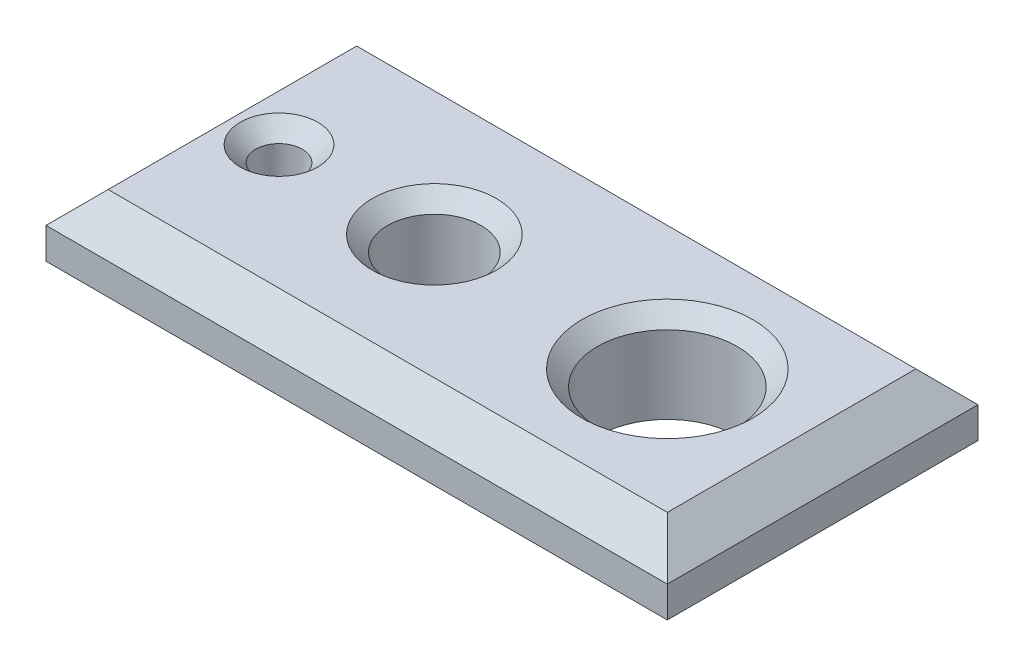
from build123d import *

# Parameters (mm, degrees)
BASE_PLATE_SKETCH_W          = 200
BASE_PLATE_SKETCH_H          = 100
BASE_PLATE_200X100X30_DEPTH  = 15
PLATE_END_CHAMFERS_10MM_SIZE = 10
PIN_HOLES_SKETCH_R           = 7.5
PIN_HOLES_SKETCH_R_2         = 15
PIN_HOLES_SKETCH_R_3         = 22.5
PIN_HOLES_15_30_45_DEPTH     = 30
PIN_HOLE_CHAMFERS_5MM_SIZE   = 5


with BuildPart() as part:
    # Base Plate Sketch → Base Plate 200x100x30 (new, symmetric)
    with BuildSketch(Plane(origin=(0, 0, 0), x_dir=(1, 0, 0), z_dir=(0, 1, 0))):
        Rectangle(BASE_PLATE_SKETCH_W, BASE_PLATE_SKETCH_H)
    extrude(amount=BASE_PLATE_200X100X30_DEPTH, both=True)

    # Plate End Chamfers 10mm
    plate_end_chamfers_10mm_edges = [part.edges().sort_by_distance(p)[0] for p in [
        (-100, 15, 0),
        (0, 15, 50),
        (100, 15, 0),
        (0, -15, 50),
        (-100, -15, 0),
        (0, -15, -50),
        (100, -15, 0),
        (0, 15, -50),
    ]]
    chamfer(plate_end_chamfers_10mm_edges, length=PLATE_END_CHAMFERS_10MM_SIZE)

    # Pin Holes Sketch → Pin Holes Ø15 Ø30 Ø45 (cut)
    with BuildSketch(Plane(origin=(0, 15, 0), x_dir=(1, 0, 0), z_dir=(0, 1, 0))):
        with Locations(Location((-75, 0, 0), (0, 0, 270))):
            Circle(PIN_HOLES_SKETCH_R)
        with Locations(Location((-25, 0, 0), (0, 0, 270))):
            Circle(PIN_HOLES_SKETCH_R_2)
        with Locations(Location((50, 0, 0), (0, 0, 270))):
            Circle(PIN_HOLES_SKETCH_R_3)
    extrude(amount=-PIN_HOLES_15_30_45_DEPTH, mode=Mode.SUBTRACT)

    # Pin Hole Chamfers 5mm
    pin_hole_chamfers_5mm_edges = [part.edges().sort_by_distance(p)[0] for p in [
        (-75, 15, -7.5),
        (-25, 15, -15),
        (50, 15, -22.5),
    ]]
    chamfer(pin_hole_chamfers_5mm_edges, length=PIN_HOLE_CHAMFERS_5MM_SIZE)


solid = part.part
